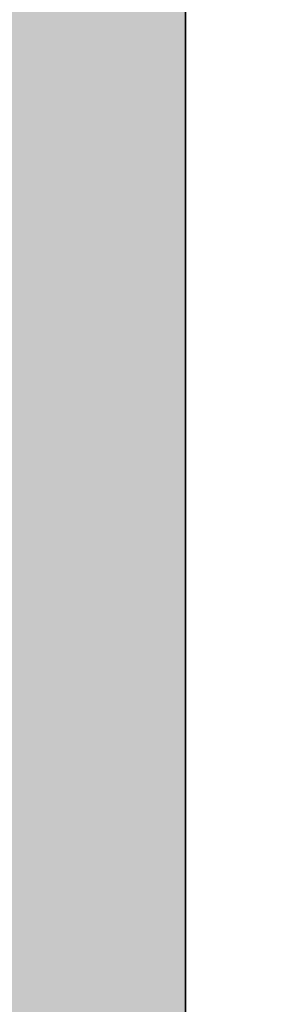
# Model space of a CAD drawing. Units: inches. Extents: x 2083 to 3317, y 1141 to 2115.
# Tile 166 of 256: x 3126.959398 to 3126.959975, y 1263.263648 to 1263.265937. Entities that reach past the tile are written whole.
import ezdxf

# ---------------------------------------------------------------- set-up
doc = ezdxf.new("R2010")
doc.units = ezdxf.units.IN
doc.layers.add('A-ANNO-DIMS', color=2, linetype='Continuous', lineweight=18)
doc.layers.add('A-WALL', color=7, linetype='Continuous', lineweight=35)
doc.layers.add('A-WALL-PATT', color=251, linetype='Continuous', lineweight=13, true_color=0x636466)
doc.styles.get("Standard").update_dxf_attribs({"font": 'arial.ttf'})
doc.dimstyles.new('ISO-25', dxfattribs={"dimtxt": 12, "dimasz": 12, "dimexe": 1.25, "dimexo": 0.625, "dimtad": 1, "dimlunit": 3, "dimtxsty": 'Standard', "dimcen": 2.5, "dimadec": 0, "dimazin": 0, "dimtfac": 1, "dimtmove": 0, "dimatfit": 3, "dimfxl": 1, "dimarcsym": 0})

# ---------------------------------------------------------------- blocks, each defined once
blk = doc.blocks.new('*D9')
at = {"layer": 'A-ANNO-DIMS', "color": 0, "lineweight": -2, "transparency": 16777216}
for p, q in [((3127.5847832, 1486.7613601), (3190.4030896, 1486.7613601)), ((3189.1530896, 1474.7613601), (3189.1530896, 1275.2613601)), ((3127.5847832, 1263.2613601), (3190.4030896, 1263.2613601))]:
    blk.add_line(p, q, dxfattribs=at)
at = {"layer": 'A-ANNO-DIMS', "color": 0, "transparency": 16777216}
for points in [[(3187.1530896, 1474.7613601), (3191.1530896, 1474.7613601), (3189.1530896, 1486.7613601)], [(3187.1530896, 1275.2613601), (3191.1530896, 1275.2613601), (3189.1530896, 1263.2613601)]]:
    blk.add_solid(points, dxfattribs=at)
at = {"layer": 'Defpoints', "color": 0, "transparency": 16777216}
for p in [(3126.9597832, 1486.7613601), (3126.9597832, 1263.2613601), (3189.1530896, 1263.2613601)]:
    blk.add_point(p, dxfattribs=at)
at = {"layer": 'A-ANNO-DIMS', "color": 0, "transparency": 16777216, "insert": (3182.4012138, 1375.0113601), "char_height": 12, "attachment_point": 5, "rotation": 90}
blk.add_mtext('18\'-7.5"', dxfattribs=at)

msp = doc.modelspace()

# ---------------------------------------------------------------- hatches: boundary and pattern name
at = {"layer": 'A-WALL-PATT'}
h = msp.add_hatch(color=256, dxfattribs=at)
h.dxf.hatch_style = 1
h.paths.add_polyline_path([(3126.9597832, 2020.7613601), (2748.9597832, 2020.7613601), (2604.9597832, 2020.7613601), (2226.9597832, 2020.7613601), (2226.9597832, 1702.7613601), (2466.9597832, 1702.7613601), (2466.9597832, 1582.7613601), (2418.9597832, 1582.7613601), (2418.9597832, 1477.7613601), (2226.9597832, 1477.7613601), (2226.9597832, 1263.2613601), (2544.9597832, 1263.2613601), (2544.9597832, 1411.7613601), (2604.9597832, 1411.7613601), (2685.9597832, 1411.7613601), (2685.9597832, 1420.7613601), (2604.9597832, 1420.7613601), (2604.9597832, 1573.7613601), (2604.9597832, 1702.7613601), (2604.9597832, 2011.7613601), (2748.9597832, 2011.7613601), (2748.9597832, 1702.7613601), (2862.9597832, 1702.7613601), (2862.9597832, 1621.7613601), (2871.9597832, 1621.7613601), (2871.9597832, 1702.7613601), (2883.9597832, 1702.7613601), (2883.9597832, 1706.9394595, -0.026459), (2883.9597832, 1711.7613601), (2757.9597832, 1711.7613601), (2757.9597832, 1807.7613601), (2787.9597832, 1807.7613601), (2787.9597832, 1812.2613601), (2757.9597832, 1812.2613601), (2757.9597832, 2011.7613601), (2877.9597832, 2011.7613601), (2877.9597832, 1812.2613601), (2847.9597832, 1812.2613601), (2847.9597832, 1807.7613601), (2889.8357425, 1807.7613601), (2889.8357425, 1812.2613601), (2882.4597832, 1812.2613601), (2882.4597832, 2011.7613601), (3117.9597832, 2011.7613601), (3117.9597832, 1812.2613601), (2937.8357425, 1812.2613601), (2937.8357425, 1807.7613601), (2995.7097832, 1807.7613601), (2995.7097832, 1796.1176655), (3000.2097832, 1796.1176655), (3000.2097832, 1807.7613601), (3117.9597832, 1807.7613601), (3117.9597832, 1711.7613601), (3000.2097832, 1711.7613601), (3000.2097832, 1760.1176655), (2998.5727047, 1760.1176655, -0.020711), (2995.7097832, 1760.1176655), (2995.7097832, 1711.7613601), (2931.9597832, 1711.7613601), (2931.9597832, 1702.7613601), (3126.9597832, 1702.7613601)])
h.paths.add_polyline_path([(2471.4597832, 2011.7613601), (2471.4597832, 1810.0113601), (2462.7169357, 1810.0113601), (2462.7169357, 1805.5113601), (2505.9597832, 1805.5113601), (2505.9597832, 1810.0113601), (2475.9597832, 1810.0113601), (2475.9597832, 2011.7613601), (2595.9597832, 2011.7613601), (2595.9597832, 1810.0113601), (2565.9597832, 1810.0113601), (2565.9597832, 1805.5113601), (2595.9597832, 1805.5113601), (2595.9597832, 1711.7613601), (2235.9597832, 1711.7613601), (2235.9597832, 1805.5113601), (2353.7097832, 1805.5113601), (2353.7097832, 1796.0541624), (2358.2097832, 1796.0541624), (2358.2097832, 1805.5113601), (2414.7169357, 1805.5113601), (2414.7169357, 1810.0113601), (2235.9597832, 1810.0113601), (2235.9597832, 2011.7613601)], flags=16)
h.paths.add_polyline_path([(2270.2047343, 1994.6100082), (2270.2047343, 1970.6100082), (2246.2047343, 1970.6100082), (2246.2047343, 1994.6100082)], flags=0)
edge = h.paths.add_edge_path(flags=0)
edge.add_ellipse((2332.027391, 1899.7981761), major_axis=(-3.0429938, 3.0429938), ratio=0.16825245, start_angle=-161.3321656, end_angle=-156.3071136, ccw=False)
edge.add_ellipse((2333.0820373, 1898.7435297), major_axis=(-1.0546463, 1.0546463), ratio=0.453532097, start_angle=-123.371019, end_angle=-94.1591066)
edge = h.paths.add_edge_path(flags=0)
edge.add_ellipse((2332.027391, 1968.8762897), major_axis=(3.0429938, 3.0429938), ratio=0.16825245, start_angle=18.6678344, end_angle=23.6928864)
edge.add_spline(control_points=[(2332.9255964, 1970.6911045), (2332.2267681, 1970.3360997), (2330.8937087, 1969.6589054), (2328.4130803, 1970.9321376), (2327.2039345, 1967.7487119), (2324.7095965, 1969.9555886), (2322.5328223, 1967.012354), (2320.0128462, 1971.2958124), (2317.6803077, 1968.1578449), (2316.0405263, 1967.1020468), (2315.4269045, 1966.8096022)], knot_values=[0, 0, 0, 0, 2.267059, 4.324559, 6.685584, 8.878641, 11.121502, 14.300359, 17.755284, 19.732645, 19.732645, 19.732645, 19.732645], degree=3, periodic=0)
edge.add_ellipse((2332.027391, 1968.8762897), major_axis=(3.0429938, 3.0429938), ratio=0.16825245, start_angle=18.6678344, end_angle=23.6928864, ccw=False)
edge.add_ellipse((2333.0820373, 1969.930936), major_axis=(1.0546463, 1.0546463), ratio=0.453532097, start_angle=56.628981, end_angle=85.8408934, ccw=False)
edge = h.paths.add_edge_path(flags=0)
edge.add_spline(control_points=[(2296.4282874, 1967.9879081), (2293.6278045, 1965.3363137), (2287.7036238, 1959.727094), (2299.7438601, 1949.9956993), (2294.5325909, 1935.6685275), (2290.5732281, 1920.6035119), (2293.3941244, 1909.9736911), (2296.1854073, 1904.9665431)], knot_values=[0.099185, 0.099185, 0.099185, 0.099185, 0.345301, 0.619822, 0.982653, 1.386093, 1.810555, 1.810555, 1.810555, 1.810555], degree=3, periodic=0)
edge.add_spline(control_points=[(2296.1854073, 1904.9665431), (2297.3835817, 1902.6193002), (2298.0009694, 1901.9493116), (2298.5529698, 1901.4681549)], knot_values=[0.006246, 0.006246, 0.006246, 0.006246, 0.055476, 0.055476, 0.055476, 0.055476], degree=3, periodic=0)
edge.add_spline(control_points=[(2298.5529698, 1901.4681549), (2297.2586121, 1900.9232238), (2295.2252939, 1900.2321257), (2293.0602287, 1900.6142053), (2292.1014227, 1900.788415), (2292.0895776, 1900.790568)], knot_values=[0.312835, 0.312835, 0.312835, 0.312835, 0.40178, 0.474987, 0.475903, 0.475903, 0.475903, 0.475903], degree=3, periodic=0)
edge.add_arc((2292.7936464, 1904.6641088), 3.9370079, 215.4208969, 259.6981795, ccw=False)
edge.add_spline(control_points=[(2289.5853139, 1902.3823039), (2289.4766524, 1902.5350874), (2289.3684805, 1902.6880353), (2289.2608648, 1902.8411699)], knot_values=[0.102872, 0.102872, 0.102872, 0.102872, 0.116896, 0.116896, 0.116896, 0.116896], degree=3, periodic=0)
edge.add_spline(control_points=[(2289.2608648, 1902.8411699), (2288.6866042, 1902.5501922), (2287.6400477, 1902.0199025), (2285.8813368, 1901.8739536), (2283.8529717, 1901.5043521), (2281.7199871, 1899.7105375), (2278.4669913, 1899.492942), (2276.1571361, 1901.8832022), (2272.2589526, 1899.8040711), (2267.7776054, 1901.8431828), (2262.2438819, 1900.1840326), (2257.414927, 1901.7820606), (2254.318374, 1900.7261196), (2253.1782849, 1900.3373431)], knot_values=[0, 0, 0, 0, 1.907977, 3.477176, 5.261074, 7.972851, 11.680248, 13.717921, 16.939592, 22.789562, 27.502503, 33.595215, 37.145618, 37.145618, 37.145618, 37.145618], degree=3, periodic=0)
edge.add_line((2253.1782849, 1900.3373431), (2250.2442397, 1902.8411699))
edge.add_line((2250.2442397, 1902.8411699), (2250.2442397, 1965.8332959))
edge.add_line((2250.2442397, 1965.8332959), (2253.1782849, 1968.3371226))
edge.add_spline(control_points=[(2253.1782849, 1968.3371226), (2254.318374, 1967.9483462), (2257.414927, 1966.8924051), (2262.2438819, 1968.4904332), (2267.7776054, 1966.8312829), (2271.5267301, 1968.5372172), (2273.8759143, 1967.8282895), (2274.2067012, 1967.7276424)], knot_values=[0, 0, 0, 0, 0.09018, 0.244935, 0.364644, 0.513233, 0.537855, 0.537855, 0.537855, 0.537855], degree=3, periodic=0)
edge.add_arc((2274.3528869, 1963.7933495), 3.9370079, 72.0511336, 92.1279492, ccw=False)
edge.add_arc((2281.2969331, 1985.2300027), 18.5962982, 252.05113361, 288.56572166)
edge.add_arc((2292.3167172, 1956.0288805), 12.6460805, 71.02678788, 113.77821843, ccw=False)
edge = h.paths.add_edge_path(flags=0)
edge.add_spline(control_points=[(2274.8994147, 1951.8561946), (2275.066156, 1951.6165924), (2275.2326866, 1951.3765878), (2275.3979871, 1951.1358545)], knot_values=[1.409916, 1.409916, 1.409916, 1.409916, 1.43159, 1.43159, 1.43159, 1.43159], degree=3, periodic=0)
edge.add_spline(control_points=[(2275.3979871, 1951.1358545), (2275.7921055, 1950.5618854), (2276.1792311, 1949.9837745), (2276.5455462, 1949.3971029)], knot_values=[1.358238, 1.358238, 1.358238, 1.358238, 1.409916, 1.409916, 1.409916, 1.409916], degree=3, periodic=0)
edge.add_line((2276.5455462, 1949.3971029), (2277.437289, 1947.8621847))
edge.add_spline(control_points=[(2277.437289, 1947.8621847), (2276.3038341, 1945.6731147), (2274.6396979, 1942.4268817), (2274.631615, 1938.0938998), (2272.7991237, 1930.8515498), (2274.3564261, 1943.8970461), (2275.9476814, 1947.9233558), (2276.5455462, 1949.3971029)], knot_values=[0.005632, 0.005632, 0.005632, 0.005632, 0.186014, 0.266002, 0.357087, 0.59639, 0.739732, 0.739732, 0.739732, 0.739732], degree=3, periodic=0)
edge.add_spline(control_points=[(2276.5455462, 1949.3971029), (2276.1792311, 1949.9837745), (2275.7921055, 1950.5618854), (2275.3979871, 1951.1358545)], knot_values=[1.358238, 1.358238, 1.358238, 1.358238, 1.409916, 1.409916, 1.409916, 1.409916], degree=3, periodic=0)
edge.add_spline(control_points=[(2275.3979871, 1951.1358545), (2274.9425002, 1950.0804523), (2274.2077604, 1948.0252718), (2273.9346018, 1944.8514774), (2272.4685341, 1937.6274891), (2273.4662155, 1945.6964663), (2274.7006154, 1951.0594725), (2274.8994147, 1951.8561946)], knot_values=[0.104364, 0.104364, 0.104364, 0.104364, 0.189636, 0.269624, 0.36071, 0.600013, 0.644622, 0.644622, 0.644622, 0.644622], degree=3, periodic=0)
h.paths.add_polyline_path([(2269.1675139, 1963.1275729, -0.357527), (2268.170633, 1960.9763695, -0.092561), (2268.170633, 1939.4363249, -0.357527), (2269.1675139, 1937.2851215, -0.357527), (2267.0163105, 1938.2820024, -0.164785), (2254.6855813, 1938.2820024, -0.357527), (2252.5343779, 1937.2851215, -0.357527), (2253.5312587, 1939.4363249, -0.092561), (2253.5312587, 1960.9763695, -0.357527), (2252.5343779, 1963.1275729, -0.357527), (2254.6855813, 1962.130692, -0.164785), (2267.0163105, 1962.130692, -0.357527)], flags=0)
h.paths.add_polyline_path([(2248.8740679, 1967.8017998), (2248.8740679, 1957.0277095), (2249.4577833, 1957.0277095), (2249.4577833, 1911.6467562), (2248.8740679, 1911.6467562), (2248.8740679, 1900.8726659), (2246.5118632, 1900.8726659, 0.197327), (2244.1496584, 1902.4568734), (2244.1496584, 1966.2175923, 0.197327), (2246.5118632, 1967.8017998)], flags=0)
h.paths.add_polyline_path([(2269.1675139, 1931.3893442, -0.357527), (2268.170633, 1929.2381408, -0.092561), (2268.170633, 1907.6980962, -0.357527), (2269.1675139, 1905.5468928, -0.357527), (2267.0163105, 1906.5437737, -0.164785), (2254.6855813, 1906.5437737, -0.357527), (2252.5343779, 1905.5468928, -0.357527), (2253.5312587, 1907.6980962, -0.092561), (2253.5312587, 1929.2381408, -0.357527), (2252.5343779, 1931.3893442, -0.357527), (2254.6855813, 1930.3924634, -0.164785), (2267.0163105, 1930.3924634, -0.357527)], flags=0)
edge = h.paths.add_edge_path(flags=0)
edge.add_spline(control_points=[(2276.1968578, 1906.7237016), (2276.1681442, 1909.0289278), (2276.1140492, 1913.371852), (2270.5984171, 1924.9249783), (2273.9051746, 1919.0127787), (2275.9217115, 1916.2620626), (2275.4745699, 1912.4021495), (2277.2578735, 1910.3806206), (2276.6960436, 1908.2250358), (2276.6462176, 1906.8130226), (2276.6178249, 1906.0084068)], knot_values=[0, 0, 0, 0, 8.61026, 16.221274, 18.843057, 23.804898, 27.440828, 29.356102, 31.203478, 33.650687, 33.650687, 33.650687, 33.650687], degree=3, periodic=0)
edge.add_spline(control_points=[(2276.6178249, 1906.0084068), (2276.6233131, 1905.6241436), (2276.4977381, 1904.6286608), (2275.4417789, 1903.8547251), (2274.9373144, 1903.0804497), (2274.8590804, 1902.8411699)], knot_values=[0.156488, 0.156488, 0.156488, 0.156488, 0.184398, 0.231376, 0.250598, 0.250598, 0.250598, 0.250598], degree=3, periodic=0)
edge.add_line((2274.8590804, 1902.8411699), (2276.50598, 1902.8411699))
edge.add_spline(control_points=[(2276.50598, 1902.8411699), (2276.7883084, 1903.0849395), (2277.6650711, 1904.1251958), (2278.2495378, 1904.340738), (2277.6538719, 1908.5273866), (2278.15567, 1906.2278078), (2278.100464, 1905.2859484), (2278.8466748, 1904.0690054), (2277.8567853, 1903.4149482), (2277.8741909, 1902.9910497), (2277.9035616, 1902.8411699)], knot_values=[0.059574, 0.059574, 0.059574, 0.059574, 0.080753, 0.103741, 0.16972, 0.176036, 0.207137, 0.240474, 0.262341, 0.27366, 0.27366, 0.27366, 0.27366], degree=3, periodic=0)
edge.add_line((2277.9035616, 1902.8411699), (2280.0298255, 1902.8411699))
edge.add_spline(control_points=[(2280.0298255, 1902.8411699), (2279.8882214, 1903.088398), (2279.4992571, 1903.9815512), (2280.1522839, 1905.9393491), (2278.103615, 1909.6577572), (2279.7623946, 1907.185285), (2280.3279002, 1904.8748608), (2280.4851086, 1903.4895904), (2281.4632687, 1903.2494323), (2281.7583431, 1902.9364967), (2281.8340361, 1902.8411699)], knot_values=[0.013856, 0.013856, 0.013856, 0.013856, 0.034874, 0.088867, 0.107879, 0.126738, 0.158714, 0.193757, 0.217487, 0.226722, 0.226722, 0.226722, 0.226722], degree=3, periodic=0)
edge.add_spline(control_points=[(2281.8340361, 1902.8411699), (2281.7875348, 1902.8267029), (2281.6470224, 1902.7829881), (2281.3955272, 1902.85949), (2281.088077, 1902.9852418), (2280.7206826, 1903.060902), (2280.3334513, 1903.0257257), (2280.1247668, 1902.898879), (2280.0298255, 1902.8411699)], knot_values=[0, 0, 0, 0, 0.14413, 0.435517, 0.749276, 1.153046, 1.548371, 1.878348, 1.878348, 1.878348, 1.878348], degree=3, periodic=0)
edge.add_line((2280.0298255, 1902.8411699), (2277.9035616, 1902.8411699))
edge.add_spline(control_points=[(2277.9035616, 1902.8411699), (2277.892855, 1902.7958553), (2277.865396, 1902.6796374), (2277.6074793, 1902.6874828), (2277.2740503, 1902.8006999), (2276.8379209, 1902.6197745), (2276.5838074, 1902.7892611), (2276.50598, 1902.8411699)], knot_values=[0, 0, 0, 0, 0.127189, 0.326199, 0.628009, 1.24357, 1.515331, 1.515331, 1.515331, 1.515331], degree=3, periodic=0)
edge.add_line((2276.50598, 1902.8411699), (2274.8590804, 1902.8411699))
edge.add_spline(control_points=[(2274.8590804, 1902.8411699), (2274.8144367, 1902.8985868), (2274.7251297, 1903.013446), (2274.4934765, 1903.1189684), (2274.2442854, 1902.9605386), (2273.9371207, 1903.1849416), (2273.6140395, 1902.9831428), (2273.4083164, 1902.8830449), (2273.322254, 1902.8411699)], knot_values=[0, 0, 0, 0, 0.21843, 0.436957, 0.687977, 0.990379, 1.398396, 1.69185, 1.69185, 1.69185, 1.69185], degree=3, periodic=0)
edge.add_spline(control_points=[(2273.322254, 1902.8411699), (2273.6167403, 1903.445692), (2274.2739977, 1904.5382529), (2276.0272387, 1904.5737017), (2276.2069634, 1906.5836372), (2276.1968578, 1906.7237016)], knot_values=[0.012227, 0.012227, 0.012227, 0.012227, 0.059472, 0.106218, 0.134458, 0.134458, 0.134458, 0.134458], degree=3, periodic=0)
h.paths.add_polyline_path([(2270.7760538, 1897.7898284), (2270.7760538, 1873.7898284), (2246.7760538, 1873.7898284), (2246.7760538, 1897.7898284)], flags=0)
h.paths.add_polyline_path([(2353.7097832, 1760.0050593), (2353.7097832, 1760.0541624), (2358.2097832, 1760.0541624, -0.033729)], flags=0)
h.paths.add_polyline_path([(2321.8191188, 1737.5291862), (2341.9953271, 1737.5291862, -0.414214), (2343.2032727, 1736.3212406), (2343.2032727, 1721.0205964, -0.414214), (2341.9953271, 1719.8126508), (2321.8191188, 1719.8126508, -0.414214), (2320.6111732, 1721.0205964), (2320.6111732, 1736.3212406, -0.414214)], flags=0)
h.paths.add_polyline_path([(2324.2350099, 1736.3212406), (2339.5794359, 1736.3212406, -0.414214), (2341.9953271, 1733.9053494), (2341.9953271, 1725.4497302, -0.414214), (2339.5794359, 1723.033839), (2333.6805885, 1723.033839), (2333.8453172, 1722.0454666, -0.870646), (2335.4253988, 1721.8258934, -0.767327), (2333.922694, 1721.4232449), (2331.2910241, 1721.4232449, -0.767327), (2329.7883193, 1721.8258934, -0.870646), (2331.3684009, 1722.0454666), (2331.5331296, 1723.033839), (2324.2350099, 1723.033839, -0.414214), (2321.8191188, 1725.4497302), (2321.8191188, 1733.9053494, -0.414214)], flags=0)
h.paths.add_polyline_path([(2570.4837892, 1928.6154443), (2589.6837892, 1928.6154443), (2590.1688286, 1928.6154443), (2590.1688286, 1904.9933971), (2570.4837892, 1904.9933971)], flags=0)
h.paths.add_polyline_path([(2574.4473242, 1927.2638215, -1), (2572.8288357, 1927.2638215, -1)], flags=0)
h.paths.add_polyline_path([(2573.0898665, 1926.9408768), (2573.925032, 1927.7760423), (2574.1477428, 1927.5533315), (2573.3125773, 1926.718166)], flags=0)
h.paths.add_polyline_path([(2578.7790648, 1919.7296175, -1), (2571.5916632, 1919.7296175, -1)], flags=0)
h.paths.add_polyline_path([(2578.385364, 1919.7296175, -1), (2571.985364, 1919.7296175, -1)], flags=0)
h.paths.add_polyline_path([(2331.5957638, 1729.4762156, -1), (2333.6179542, 1729.4762156, -1)], flags=0)
h.paths.add_polyline_path([(2578.0342282, 1927.2638215, -1), (2576.4157396, 1927.2638215, -1)], flags=0)
h.paths.add_polyline_path([(2576.6888513, 1927.5310886), (2576.9115621, 1927.7537993), (2577.7467276, 1926.9186339), (2577.5240168, 1926.6959231)], flags=0)
h.paths.add_polyline_path([(2578.1390648, 1909.8595388, -1), (2572.2316632, 1909.8595388, -1)], flags=0)
h.paths.add_polyline_path([(2577.745364, 1909.8595388, -1), (2572.625364, 1909.8595388, -1)], flags=0)
h.paths.add_polyline_path([(2583.7977179, 1927.2638215, -1), (2582.1792294, 1927.2638215, -1)], flags=0)
h.paths.add_polyline_path([(2582.7186487, 1927.7537993), (2583.5538142, 1926.9186339), (2583.3311034, 1926.6959231), (2582.4959379, 1927.5310886)], flags=0)
h.paths.add_polyline_path([(2582.4959379, 1927.5310886), (2582.7186487, 1927.7537993), (2583.5538142, 1926.9186339), (2583.3311034, 1926.6959231)], flags=0)
h.paths.add_polyline_path([(2587.7390648, 1920.5296175, -1), (2581.8316632, 1920.5296175, -1)], flags=0)
h.paths.add_polyline_path([(2587.345364, 1920.5296175, -1), (2582.225364, 1920.5296175, -1)], flags=0)
h.paths.add_polyline_path([(2587.3846219, 1927.2638215, -1), (2585.7661333, 1927.2638215, -1)], flags=0)
h.paths.add_polyline_path([(2586.0819925, 1926.9802469), (2586.917158, 1927.8154124), (2587.1398688, 1927.5927016), (2586.3047033, 1926.7575361)], flags=0)
h.paths.add_polyline_path([(2588.3790648, 1910.6595388, -1), (2581.1916632, 1910.6595388, -1)], flags=0)
h.paths.add_polyline_path([(2587.985364, 1910.6595388, -1), (2581.585364, 1910.6595388, -1)], flags=0)
h.paths.add_polyline_path([(2417.1677288, 1729.4778955), (2437.3439372, 1729.4778955, -0.414214), (2438.5518828, 1728.2699499), (2438.5518828, 1712.9693057, -0.414214), (2437.3439372, 1711.7613601), (2417.1677288, 1711.7613601, -0.414214), (2415.9597832, 1712.9693057), (2415.9597832, 1728.2699499, -0.414214)], flags=0)
h.paths.add_polyline_path([(2419.58362, 1728.2699499), (2434.928046, 1728.2699499, -0.414214), (2437.3439372, 1725.8540587), (2437.3439372, 1717.3984395, -0.414214), (2434.928046, 1714.9825483), (2429.0291985, 1714.9825483), (2429.1939273, 1713.9941758, -0.870646), (2430.7740089, 1713.7746027, -0.767327), (2429.2713041, 1713.3719542), (2426.6396342, 1713.3719542, -0.767327), (2425.1369294, 1713.7746027, -0.870646), (2426.717011, 1713.9941758), (2426.8817397, 1714.9825483), (2419.58362, 1714.9825483, -0.414214), (2417.1677288, 1717.3984395), (2417.1677288, 1725.8540587, -0.414214)], flags=0)
h.paths.add_polyline_path([(2419.58362, 1728.2699499), (2434.928046, 1728.2699499, -0.414214), (2437.3439372, 1725.8540587), (2437.3439372, 1717.3984395, -0.414214), (2434.928046, 1714.9825483), (2429.0291985, 1714.9825483), (2428.3581177, 1719.0090337), (2427.5528206, 1719.0090337), (2426.8817397, 1714.9825483), (2419.58362, 1714.9825483, -0.414214), (2417.1677288, 1717.3984395), (2417.1677288, 1725.8540587, -0.414214)], flags=0)
h.paths.add_polyline_path([(2426.9443739, 1721.4249248, -1), (2428.9665643, 1721.4249248, -1)], flags=0)
h.paths.add_polyline_path([(2475.9597832, 1702.7613601), (2595.9597832, 1702.7613601), (2595.9597832, 1582.7613601), (2475.9597832, 1582.7613601)], flags=16)
h.paths.add_polyline_path([(2427.9597832, 1573.7613601), (2595.9597832, 1573.7613601), (2595.9597832, 1468.7613601), (2595.9597832, 1420.7613601), (2384.4597832, 1420.7613601), (2384.4597832, 1468.7613601), (2427.9597832, 1468.7613601)], flags=16)
h.paths.add_polyline_path([(2379.9597832, 1468.7613601), (2379.9597832, 1420.7613601), (2235.9597832, 1420.7613601), (2235.9597832, 1468.7613601)], flags=16)
h.paths.add_polyline_path([(2317.8159962, 1466.695767), (2337.9922045, 1466.695767, -0.414214), (2339.2001501, 1465.4878214), (2339.2001501, 1450.1871771, -0.414214), (2337.9922045, 1448.9792315), (2317.8159962, 1448.9792315, -0.414214), (2316.6080506, 1450.1871771), (2316.6080506, 1465.4878214, -0.414214)], flags=0)
h.paths.add_polyline_path([(2320.2318874, 1465.4878214), (2335.5763133, 1465.4878214, -0.414214), (2337.9922045, 1463.0719302), (2337.9922045, 1454.616311, -0.414214), (2335.5763133, 1452.2004198), (2329.6774659, 1452.2004198), (2329.8421946, 1451.2120473, -0.870646), (2331.4222762, 1450.9924742, -0.767327), (2329.9195714, 1450.5898257), (2327.2879015, 1450.5898257, -0.767327), (2325.7851967, 1450.9924742, -0.870646), (2327.3652783, 1451.2120473), (2327.530007, 1452.2004198), (2320.2318874, 1452.2004198, -0.414214), (2317.8159962, 1454.616311), (2317.8159962, 1463.0719302, -0.414214)], flags=0)
h.paths.add_polyline_path([(2320.2318874, 1465.4878214), (2335.5763133, 1465.4878214, -0.414214), (2337.9922045, 1463.0719302), (2337.9922045, 1454.616311, -0.414214), (2335.5763133, 1452.2004198), (2329.6774659, 1452.2004198), (2329.006385, 1456.2269051), (2328.2010879, 1456.2269051), (2327.530007, 1452.2004198), (2320.2318874, 1452.2004198, -0.414214), (2317.8159962, 1454.616311), (2317.8159962, 1463.0719302, -0.414214)], flags=0)
h.paths.add_polyline_path([(2327.5926413, 1458.6427963, -1), (2329.6148317, 1458.6427963, -1)], flags=0)
h.paths.add_polyline_path([(2244.4117436, 1433.3404531), (2241.9209449, 1433.3404531, -0.414214), (2240.0178562, 1435.2435418), (2240.0178562, 1440.9528078, -0.414211), (2241.920925, 1442.8558965), (2244.4117436, 1442.8558965, -1.976472)], flags=0)
h.paths.add_polyline_path([(2245.3568884, 1434.3975358, -0.414214), (2245.3568884, 1441.7988138, -2.144098)], flags=0)
h.paths.add_polyline_path([(2535.9597832, 1416.2613601), (2535.9597832, 1272.2613601), (2235.9597832, 1272.2613601), (2235.9597832, 1416.2613601)], flags=16)
h.paths.add_polyline_path([(2260.1195614, 1384.2928413), (2260.1195614, 1362.0386487), (2237.8653688, 1362.0386487), (2237.8653688, 1384.2928413)], flags=0)
edge = h.paths.add_edge_path(flags=0)
edge.add_line((2318.2518466, 1362.0932983), (2318.1457968, 1362.0009726))
edge.add_ellipse((2317.4451158, 1360.4310442), major_axis=(2.8216404, 2.8216404), ratio=0.16825245, start_angle=18.6678344, end_angle=20.9481273, ccw=False)
edge.add_ellipse((2318.4230451, 1361.4089735), major_axis=(0.9779293, 0.9779293), ratio=0.453532097, start_angle=56.628981, end_angle=70.2262012, ccw=False)
edge = h.paths.add_edge_path(flags=0)
edge.add_line((2319.1073699, 1295.5710784), (2319.0150442, 1295.6771282))
edge.add_ellipse((2317.4451158, 1296.3778091), major_axis=(-2.8216404, 2.8216404), ratio=0.16825245, start_angle=-161.3321656, end_angle=-159.0518727, ccw=False)
edge.add_ellipse((2318.4230451, 1295.3998798), major_axis=(-0.9779293, 0.9779293), ratio=0.453532097, start_angle=-123.371019, end_angle=-109.7737988)
edge = h.paths.add_edge_path(flags=0)
edge.add_spline(control_points=[(2284.2103489, 1301.1702189), (2284.5806878, 1300.444719), (2284.8911891, 1299.8920243), (2285.159553, 1299.4610182)], knot_values=[0.039066, 0.039066, 0.039066, 0.039066, 0.055476, 0.055476, 0.055476, 0.055476], degree=3, periodic=0)
edge.add_line((2285.159553, 1299.4610182), (2284.2103489, 1301.1702189))
edge = h.paths.add_edge_path(flags=0)
edge.add_line((2280.4124579, 1297.2980125), (2283.3699905, 1297.0361216))
edge.add_line((2283.3699905, 1297.0361216), (2286.4056902, 1297.9263104))
edge.add_spline(control_points=[(2286.4056902, 1297.9263104), (2285.305487, 1297.4631193), (2284.3447774, 1297.1291508), (2283.3699905, 1297.0361216)], knot_values=[0.394369, 0.394369, 0.394369, 0.394369, 0.475903, 0.475903, 0.475903, 0.475903], degree=3, periodic=0)
edge.add_spline(control_points=[(2283.3699905, 1297.0361216), (2283.2813895, 1297.027666), (2282.316289, 1296.9573356), (2281.3125019, 1297.1344787), (2280.4234414, 1297.2960161), (2280.4124579, 1297.2980125)], knot_values=[0.312835, 0.312835, 0.312835, 0.312835, 0.320246, 0.393453, 0.394369, 0.394369, 0.394369, 0.394369], degree=3, periodic=0)
edge = h.paths.add_edge_path(flags=0)
edge.add_line((2284.4355615, 1359.6072854), (2280.4462909, 1355.328047))
edge.add_line((2280.4462909, 1355.328047), (2279.5799868, 1351.0177544))
edge.add_line((2279.5799868, 1351.0177544), (2282.4129737, 1346.5804327))
edge.add_spline(control_points=[(2282.4129737, 1346.5804327), (2283.1533308, 1345.5892358), (2284.2528957, 1344.0288973), (2284.801037, 1342.3871671), (2284.9351625, 1341.8055443)], knot_values=[1.240098, 1.240098, 1.240098, 1.240098, 1.332892, 1.382712, 1.382712, 1.382712, 1.382712], degree=3, periodic=0)
edge.add_spline(control_points=[(2284.9351625, 1341.8055443), (2285.3191079, 1340.1406002), (2285.2330291, 1338.4092041), (2284.9099384, 1336.6541222)], knot_values=[1.097484, 1.097484, 1.097484, 1.097484, 1.240098, 1.240098, 1.240098, 1.240098], degree=3, periodic=0)
edge.add_spline(control_points=[(2284.9099384, 1336.6541222), (2284.5868478, 1334.8990403), (2284.0267453, 1333.1202725), (2283.4626437, 1331.3605849)], knot_values=[0.95487, 0.95487, 0.95487, 0.95487, 1.097484, 1.097484, 1.097484, 1.097484], degree=3, periodic=0)
edge.add_line((2283.4626437, 1331.3605849), (2281.8903759, 1326.153357))
edge.add_line((2281.8903759, 1326.153357), (2280.7562592, 1321.0560888))
edge.add_line((2280.7562592, 1321.0560888), (2280.2992048, 1316.0019772))
edge.add_line((2280.2992048, 1316.0019772), (2280.7159327, 1310.9500678))
edge.add_line((2280.7159327, 1310.9500678), (2282.0280939, 1305.9721367))
edge.add_line((2282.0280939, 1305.9721367), (2284.2103489, 1301.1702189))
edge.add_spline(control_points=[(2284.2103489, 1301.1702189), (2283.3407305, 1302.7301854), (2282.6119044, 1304.3364933), (2282.0280939, 1305.9721367)], knot_values=[0.099185, 0.099185, 0.099185, 0.099185, 0.241799, 0.241799, 0.241799, 0.241799], degree=3, periodic=0)
edge.add_spline(control_points=[(2282.0280939, 1305.9721367), (2281.4442835, 1307.6077801), (2281.0054886, 1309.2727591), (2280.7159327, 1310.9500678)], knot_values=[0.241799, 0.241799, 0.241799, 0.241799, 0.384413, 0.384413, 0.384413, 0.384413], degree=3, periodic=0)
edge.add_spline(control_points=[(2280.7159327, 1310.9500678), (2280.4332411, 1312.5876134), (2280.2893863, 1314.2769594), (2280.2988938, 1315.9620324), (2280.2992048, 1316.0019772)], knot_values=[0.384413, 0.384413, 0.384413, 0.384413, 0.523647, 0.527028, 0.527028, 0.527028, 0.527028], degree=3, periodic=0)
edge.add_spline(control_points=[(2280.2992048, 1316.0019772), (2280.3123257, 1317.6869552), (2280.4778706, 1319.3679256), (2280.7562592, 1321.0560888)], knot_values=[0.527028, 0.527028, 0.527028, 0.527028, 0.669642, 0.669642, 0.669642, 0.669642], degree=3, periodic=0)
edge.add_spline(control_points=[(2280.7562592, 1321.0560888), (2281.0346478, 1322.7442519), (2281.4258801, 1324.4396079), (2281.8903759, 1326.153357)], knot_values=[0.669642, 0.669642, 0.669642, 0.669642, 0.812256, 0.812256, 0.812256, 0.812256], degree=3, periodic=0)
edge.add_spline(control_points=[(2281.8903759, 1326.153357), (2282.2643834, 1327.5332507), (2282.7878702, 1329.2618097), (2283.352751, 1331.0177803), (2283.4626437, 1331.3605849)], knot_values=[0.812256, 0.812256, 0.812256, 0.812256, 0.927087, 0.95487, 0.95487, 0.95487, 0.95487], degree=3, periodic=0)
edge.add_line((2283.4626437, 1331.3605849), (2284.9099384, 1336.6541222))
edge.add_line((2284.9099384, 1336.6541222), (2284.9351625, 1341.8055443))
edge.add_line((2284.9351625, 1341.8055443), (2282.4129737, 1346.5804327))
edge.add_spline(control_points=[(2282.4129737, 1346.5804327), (2281.2751273, 1348.1037918), (2280.0784467, 1349.5703178), (2279.5799868, 1351.0177544)], knot_values=[1.382712, 1.382712, 1.382712, 1.382712, 1.525326, 1.525326, 1.525326, 1.525326], degree=3, periodic=0)
edge.add_spline(control_points=[(2279.5799868, 1351.0177544), (2279.4432818, 1351.4147209), (2279.1363124, 1352.856922), (2279.7351897, 1354.2903851), (2280.4462909, 1355.328047)], knot_values=[1.525326, 1.525326, 1.525326, 1.525326, 1.564439, 1.667941, 1.667941, 1.667941, 1.667941], degree=3, periodic=0)
edge.add_spline(control_points=[(2280.4462909, 1355.328047), (2281.4261132, 1356.7578354), (2282.9308373, 1358.1825604), (2284.4355615, 1359.6072854)], knot_values=[1.667941, 1.667941, 1.667941, 1.667941, 1.810555, 1.810555, 1.810555, 1.810555], degree=3, periodic=0)
edge.add_arc((2280.6230749, 1348.518181), 11.7261796, 71.02678788, 113.77821843)
edge.add_arc((2270.4048917, 1375.5951559), 17.2435667, 252.05113361, 288.56572166, ccw=False)
edge.add_arc((2263.9659692, 1355.7178471), 3.6506221, 72.0511336, 92.1279492)
edge.add_arc((2263.9659692, 1355.7178471), 3.6506221, 92.1279492, 177.98513)
edge.add_spline(control_points=[(2260.3176041, 1355.8461989), (2260.2604169, 1354.2206683), (2260.551278, 1350.1865469), (2262.9993445, 1346.7662507), (2264.4727415, 1344.6490245)], knot_values=[1.43159, 1.43159, 1.43159, 1.43159, 1.564144, 1.770695, 1.770695, 1.770695, 1.770695], degree=3, periodic=0)
edge.add_line((2264.4727415, 1344.6490245), (2264.9355904, 1343.9825301))
edge.add_spline(control_points=[(2263.8010444, 1340.2481052), (2263.8432379, 1340.5140884), (2264.0672444, 1341.7564652), (2264.5126928, 1343.0024532), (2264.9350468, 1343.9810834)], knot_values=[0.53657, 0.53657, 0.53657, 0.53657, 0.559349, 0.644622, 0.644622, 0.644622, 0.644622], degree=3, periodic=0)
edge.add_spline(control_points=[(2264.9350468, 1343.9810834), (2265.1177715, 1343.7149747), (2265.2988751, 1343.4479058), (2265.4767562, 1343.1793646)], knot_values=[1.384077, 1.384077, 1.384077, 1.384077, 1.409916, 1.409916, 1.409916, 1.409916], degree=3, periodic=0)
edge.add_spline(control_points=[(2265.4767562, 1343.1793646), (2265.6546373, 1342.9108234), (2265.8292958, 1342.64081), (2265.9991301, 1342.368812)], knot_values=[1.358238, 1.358238, 1.358238, 1.358238, 1.384077, 1.384077, 1.384077, 1.384077], degree=3, periodic=0)
edge.add_line((2265.9991301, 1342.368812), (2266.8260057, 1340.9455468))
edge.add_spline(control_points=[(2266.8260057, 1340.9455468), (2268.894401, 1337.0896912), (2271.3981727, 1325.8430009), (2270.5161644, 1310.5685568), (2275.9193759, 1301.860609), (2277.7895113, 1299.1994495)], knot_values=[0.116896, 0.116896, 0.116896, 0.116896, 0.472987, 1.050969, 1.313793, 1.313793, 1.313793, 1.313793], degree=3, periodic=0)
edge.add_spline(control_points=[(2277.7895113, 1299.1994495), (2277.8394051, 1299.1284519), (2277.8894277, 1299.0574975), (2277.9395717, 1298.9865839)], knot_values=[0.109884, 0.109884, 0.109884, 0.109884, 0.116896, 0.116896, 0.116896, 0.116896], degree=3, periodic=0)
edge.add_line((2277.9395717, 1298.9865839), (2277.7888489, 1299.1991139))
edge.add_spline(control_points=[(2277.7888489, 1299.1991139), (2277.2565819, 1298.9294144), (2276.2863504, 1298.4379024), (2275.0393517, 1298.3344186), (2274.3833299, 1298.2388951), (2274.2152543, 1298.209338)], knot_values=[33.12187, 33.12187, 33.12187, 33.12187, 35.029056, 36.598255, 37.144827, 37.144827, 37.144827, 37.144827], degree=3, periodic=0)
edge.add_line((2274.2152543, 1298.209338), (2273.073147, 1297.8929607))
edge.add_spline(control_points=[(2273.073147, 1297.8929607), (2272.3229363, 1297.579784), (2271.0391507, 1296.5105078), (2269.2483948, 1296.2260622), (2268.4231004, 1296.3746543)], knot_values=[26.532584, 26.532584, 26.532584, 26.532584, 29.198919, 31.839101, 31.839101, 31.839101, 31.839101], degree=3, periodic=0)
edge.add_line((2268.4231004, 1296.3746543), (2263.8785014, 1297.4575338))
edge.add_spline(control_points=[(2263.8785014, 1297.4575338), (2263.5560769, 1297.3594345), (2261.8603064, 1296.8386943), (2260.2387805, 1297.2824073), (2258.9334543, 1297.5164611)], knot_values=[15.919551, 15.919551, 15.919551, 15.919551, 16.939592, 21.226067, 21.226067, 21.226067, 21.226067], degree=3, periodic=0)
edge.add_line((2258.9334543, 1297.5164611), (2254.0552332, 1297.3290098))
edge.add_spline(control_points=[(2254.0552332, 1297.3290098), (2253.7555255, 1297.295815), (2252.1136834, 1297.1651738), (2250.4618687, 1297.5442209), (2249.1296862, 1297.6678818)], knot_values=[5.306517, 5.306517, 5.306517, 5.306517, 6.276435, 10.613034, 10.613034, 10.613034, 10.613034], degree=3, periodic=0)
edge.add_line((2249.1296862, 1297.6678818), (2244.3316495, 1296.8777561))
edge.add_line((2244.3316495, 1296.8777561), (2241.6110326, 1299.1994495))
edge.add_line((2241.6110326, 1299.1994495), (2241.6110326, 1357.6094038))
edge.add_line((2241.6110326, 1357.6094038), (2244.3316495, 1359.9310973))
edge.add_line((2244.3316495, 1359.9310973), (2252.7288228, 1359.5426917))
edge.add_spline(control_points=[(2252.7288228, 1359.5426917), (2252.8709387, 1359.5464396), (2253.3057402, 1359.5481716), (2253.7398447, 1359.5142744), (2254.0317419, 1359.4824261)], knot_values=[0.233291, 0.233291, 0.233291, 0.233291, 0.244935, 0.268927, 0.268927, 0.268927, 0.268927], degree=3, periodic=0)
edge.add_line((2254.0317419, 1359.4824261), (2259.5871899, 1359.4163899))
edge.add_spline(control_points=[(2259.5871899, 1359.4163899), (2260.6770676, 1359.6285026), (2262.0731971, 1359.8970025), (2263.5236925, 1359.4592776), (2263.8304173, 1359.3659518)], knot_values=[0.422516, 0.422516, 0.422516, 0.422516, 0.513233, 0.537855, 0.537855, 0.537855, 0.537855], degree=3, periodic=0)
edge.add_arc((2263.9659692, 1355.7178471), 3.6506221, 72.0511336, 92.1279492, ccw=False)
edge.add_arc((2270.4048917, 1375.5951559), 17.2435667, 252.05113361, 288.56572166)
edge.add_arc((2280.6230749, 1348.518181), 11.7261796, 71.02678788, 113.77821843, ccw=False)
h.paths.add_polyline_path([(2240.3405298, 1359.4347149), (2240.3405298, 1349.4443532), (2240.8817846, 1349.4443532), (2240.8817846, 1307.3645001), (2240.3405298, 1307.3645001), (2240.3405298, 1297.3741385), (2238.1501565, 1297.3741385, 0.197327), (2235.9597832, 1298.8431076), (2235.9597832, 1357.9657458, 0.197327), (2238.1501565, 1359.4347149)], flags=0)
h.paths.add_polyline_path([(2259.1577904, 1355.1005005, -0.357527), (2258.2334246, 1353.1057799, -0.092561), (2258.2334246, 1333.1326007, -0.357527), (2259.1577904, 1331.1378801, -0.357527), (2257.1630698, 1332.0622458, -0.164785), (2245.7293022, 1332.0622458, -0.357527), (2243.7345816, 1331.1378801, -0.357527), (2244.6589474, 1333.1326007, -0.092561), (2244.6589474, 1353.1057799, -0.357527), (2243.7345816, 1355.1005005, -0.357527), (2245.7293022, 1354.1761347, -0.164785), (2257.1630698, 1354.1761347, -0.357527)], flags=0)
edge = h.paths.add_edge_path(flags=0)
edge.add_line((2265.9991301, 1342.368812), (2266.8260057, 1340.9455468))
edge.add_line((2266.8260057, 1340.9455468), (2265.3075567, 1337.8140664))
edge.add_line((2265.3075567, 1337.8140664), (2264.358232, 1334.6529388))
edge.add_line((2264.358232, 1334.6529388), (2264.2620123, 1333.7997046))
edge.add_spline(control_points=[(2264.2620123, 1333.7997046), (2264.2083565, 1333.187055), (2264.1620602, 1332.3655252), (2264.0071444, 1331.4139326), (2263.9690487, 1331.2018338)], knot_values=[0.464444, 0.464444, 0.464444, 0.464444, 0.516691, 0.531608, 0.531608, 0.531608, 0.531608], degree=3, periodic=0)
edge.add_spline(control_points=[(2263.9690487, 1331.2018338), (2263.7745349, 1330.1188727), (2263.4243703, 1328.7908386), (2263.2574202, 1328.5306516), (2263.2340282, 1328.5146115)], knot_values=[0.372682, 0.372682, 0.372682, 0.372682, 0.44885, 0.464444, 0.464444, 0.464444, 0.464444], degree=3, periodic=0)
edge.add_spline(control_points=[(2263.2340282, 1328.5146115), (2263.096382, 1328.4202271), (2263.1311696, 1329.3014765), (2263.2749528, 1330.6157493)], knot_values=[0.280919, 0.280919, 0.280919, 0.280919, 0.372682, 0.372682, 0.372682, 0.372682], degree=3, periodic=0)
edge.add_spline(control_points=[(2263.2749528, 1330.6157493), (2263.4187361, 1331.930022), (2263.6715151, 1333.677318), (2263.9698519, 1335.3150268)], knot_values=[0.189157, 0.189157, 0.189157, 0.189157, 0.280919, 0.280919, 0.280919, 0.280919], degree=3, periodic=0)
edge.add_spline(control_points=[(2263.9698519, 1335.3150268), (2264.1004958, 1336.0321917), (2264.4187827, 1337.6219113), (2264.7548476, 1338.8644304), (2264.9474193, 1339.4911244)], knot_values=[0.097394, 0.097394, 0.097394, 0.097394, 0.137578, 0.189157, 0.189157, 0.189157, 0.189157], degree=3, periodic=0)
edge.add_spline(control_points=[(2264.9474193, 1339.4911244), (2265.2900171, 1340.6060546), (2265.6442376, 1341.4939958), (2265.9991301, 1342.368812)], knot_values=[0.005632, 0.005632, 0.005632, 0.005632, 0.097394, 0.097394, 0.097394, 0.097394], degree=3, periodic=0)
h.paths.add_polyline_path([(2259.1577904, 1325.6709733, -0.357527), (2258.2334246, 1323.6762527, -0.092561), (2258.2334246, 1303.7030735, -0.357527), (2259.1577904, 1301.7083529, -0.357527), (2257.1630698, 1302.6327186, -0.164785), (2245.7293022, 1302.6327186, -0.357527), (2243.7345816, 1301.7083529, -0.357527), (2244.6589474, 1303.7030735, -0.092561), (2244.6589474, 1323.6762527, -0.357527), (2243.7345816, 1325.6709733, -0.357527), (2245.7293022, 1324.7466075, -0.164785), (2257.1630698, 1324.7466075, -0.357527)], flags=0)
edge = h.paths.add_edge_path(flags=0)
edge.add_spline(control_points=[(2261.7089377, 1317.3114208), (2261.6794818, 1317.4175798), (2261.7618581, 1317.3885347), (2262.4907358, 1316.0898725), (2262.962185, 1315.3008975)], knot_values=[14.955861, 14.955861, 14.955861, 14.955861, 16.221274, 18.694826, 18.694826, 18.694826, 18.694826], degree=3, periodic=0)
edge.add_spline(control_points=[(2262.962185, 1315.3008975), (2262.9904374, 1315.2536169), (2263.7020958, 1314.0673762), (2264.3489834, 1313.1271533), (2264.7300545, 1312.1641544)], knot_values=[18.694826, 18.694826, 18.694826, 18.694826, 18.843057, 22.433791, 22.433791, 22.433791, 22.433791], degree=3, periodic=0)
edge.add_spline(control_points=[(2264.7300545, 1312.1641544), (2264.8755649, 1311.7964373), (2265.1768733, 1310.7698073), (2265.1430689, 1309.5592623), (2265.2477363, 1308.8241926)], knot_values=[22.433791, 22.433791, 22.433791, 22.433791, 23.804898, 26.172756, 26.172756, 26.172756, 26.172756], degree=3, periodic=0)
edge.add_line((2265.2477363, 1308.8241926), (2265.8507741, 1307.1718879))
edge.add_spline(control_points=[(2265.8507741, 1307.1718879), (2266.0650246, 1306.8216779), (2266.3843872, 1306.3322461), (2266.4244001, 1305.7805489), (2266.4203688, 1305.6112163)], knot_values=[28.062562, 28.062562, 28.062562, 28.062562, 29.356102, 29.911721, 29.911721, 29.911721, 29.911721], degree=3, periodic=0)
edge.add_spline(control_points=[(2266.4203688, 1305.6112163), (2266.4161162, 1305.4325896), (2266.393999, 1305.2499979), (2266.3647773, 1305.0658571)], knot_values=[29.911721, 29.911721, 29.911721, 29.911721, 30.497837, 30.497837, 30.497837, 30.497837], degree=3, periodic=0)
edge.add_line((2266.3647773, 1305.0658571), (2266.0661511, 1302.1362954))
edge.add_spline(control_points=[(2266.0661511, 1302.1362954), (2266.0712401, 1301.7799843), (2265.9980761, 1301.1999847), (2265.6632664, 1300.7589613), (2265.5089084, 1300.5858824)], knot_values=[0.156488, 0.156488, 0.156488, 0.156488, 0.184398, 0.203543, 0.203543, 0.203543, 0.203543], degree=3, periodic=0)
edge.add_line((2265.5089084, 1300.5858824), (2264.4353411, 1299.1994495))
edge.add_line((2264.4353411, 1299.1994495), (2265.962442, 1299.1994495))
edge.add_line((2265.962442, 1299.1994495), (2267.3359898, 1301.1752758))
edge.add_line((2267.3359898, 1301.1752758), (2267.3116668, 1301.9862366))
edge.add_spline(control_points=[(2267.3116668, 1301.9862366), (2267.261111, 1302.8623959), (2267.1602121, 1303.7371316), (2267.2714865, 1303.3258962)], knot_values=[0.126229, 0.126229, 0.126229, 0.126229, 0.166617, 0.166617, 0.166617, 0.166617], degree=3, periodic=0)
edge.add_spline(control_points=[(2267.2714865, 1303.3258962), (2267.2800347, 1303.2943047), (2267.3097851, 1303.1753659), (2267.3734504, 1302.8836084), (2267.4061233, 1302.6828291), (2267.4179259, 1302.6010251)], knot_values=[0.166617, 0.166617, 0.166617, 0.166617, 0.16972, 0.176036, 0.180765, 0.180765, 0.180765, 0.180765], degree=3, periodic=0)
edge.add_spline(control_points=[(2267.7438914, 1300.9875045), (2267.6875832, 1301.1509426), (2267.4805198, 1301.6566644), (2267.4837514, 1302.1447877), (2267.4179259, 1302.6010251)], knot_values=[0.180765, 0.180765, 0.180765, 0.180765, 0.193767, 0.220139, 0.220139, 0.220139, 0.220139], degree=3, periodic=0)
edge.add_line((2267.4179259, 1302.6010251), (2267.7438914, 1300.9875045))
edge.add_spline(control_points=[(2267.7438914, 1300.9875045), (2267.8319608, 1300.7318778), (2267.9320205, 1300.3099042), (2267.5548409, 1299.9745185), (2267.429366, 1299.8292073)], knot_values=[0.220139, 0.220139, 0.220139, 0.220139, 0.240474, 0.25489, 0.25489, 0.25489, 0.25489], degree=3, periodic=0)
edge.add_line((2267.429366, 1299.8292073), (2267.2583608, 1299.1994495))
edge.add_line((2267.2583608, 1299.1994495), (2269.229956, 1299.1994495))
edge.add_spline(control_points=[(2269.229956, 1299.1994495), (2269.0986525, 1299.4286938), (2268.842774, 1300.0162509), (2269.0115749, 1300.9159235), (2268.9467957, 1301.6607397)], knot_values=[0.013856, 0.013856, 0.013856, 0.013856, 0.034874, 0.067073, 0.067073, 0.067073, 0.067073], degree=3, periodic=0)
edge.add_line((2268.9467957, 1301.6607397), (2268.4315815, 1303.6031089))
edge.add_spline(control_points=[(2268.4315815, 1303.6031089), (2268.1755957, 1304.1923747), (2267.5962136, 1305.2512977), (2268.0406981, 1304.6232098), (2268.2513938, 1304.2824205)], knot_values=[0.090155, 0.090155, 0.090155, 0.090155, 0.107879, 0.120289, 0.120289, 0.120289, 0.120289], degree=3, periodic=0)
edge.add_spline(control_points=[(2268.2513938, 1304.2824205), (2268.3608818, 1304.1053294), (2269.0577527, 1302.9179833), (2269.382691, 1301.5904186), (2269.5214051, 1300.7759312), (2269.5752202, 1300.5557836)], knot_values=[0.120289, 0.120289, 0.120289, 0.120289, 0.126738, 0.158714, 0.173506, 0.173506, 0.173506, 0.173506], degree=3, periodic=0)
edge.add_line((2269.5752202, 1300.5557836), (2270.6857984, 1299.4212579))
edge.add_spline(control_points=[(2270.6857984, 1299.4212579), (2270.7672206, 1299.3572512), (2270.8378523, 1299.2814011), (2270.9029248, 1299.1994495)], knot_values=[0.21816, 0.21816, 0.21816, 0.21816, 0.226722, 0.226722, 0.226722, 0.226722], degree=3, periodic=0)
edge.add_line((2270.9372012, 1299.1929131), (2270.9029248, 1299.1994495))
edge.add_spline(control_points=[(2270.9029248, 1299.1994495), (2270.8598061, 1299.1860349), (2270.7295148, 1299.1455), (2270.4963139, 1299.216437), (2270.2716612, 1299.3083234), (2270.1210168, 1299.3479612), (2270.0633386, 1299.3595566)], knot_values=[0.939174, 0.939174, 0.939174, 0.939174, 1.083304, 1.374691, 1.68845, 1.878348, 1.878348, 1.878348, 1.878348], degree=3, periodic=0)
edge.add_line((2270.0633386, 1299.3595566), (2269.229956, 1299.1994495))
edge.add_line((2269.229956, 1299.1994495), (2267.2583608, 1299.1994495))
edge.add_spline(control_points=[(2267.2583608, 1299.1994495), (2267.248433, 1299.1574312), (2267.2229714, 1299.0496673), (2266.9838161, 1299.056942), (2266.8092097, 1299.1162303), (2266.6769047, 1299.1090913), (2266.636531, 1299.1048147)], knot_values=[0.757665, 0.757665, 0.757665, 0.757665, 0.884854, 1.083864, 1.385675, 1.515331, 1.515331, 1.515331, 1.515331], degree=3, periodic=0)
edge.add_spline(control_points=[(2266.636531, 1299.1048147), (2266.4852248, 1299.0887878), (2266.2358066, 1299.0171229), (2266.0346081, 1299.1513168), (2265.962442, 1299.1994495)], knot_values=[0, 0, 0, 0, 0.485905, 0.757665, 0.757665, 0.757665, 0.757665], degree=3, periodic=0)
edge.add_line((2265.962442, 1299.1994495), (2264.4353411, 1299.1994495))
edge.add_line((2264.4353411, 1299.1994495), (2263.8584442, 1299.3671176))
edge.add_spline(control_points=[(2263.8584442, 1299.3671176), (2263.8189433, 1299.3709053), (2263.7795277, 1299.3857212), (2263.7401308, 1299.4015039)], knot_values=[0.845925, 0.845925, 0.845925, 0.845925, 0.978627, 0.978627, 0.978627, 0.978627], degree=3, periodic=0)
edge.add_line((2263.7217862, 1299.3964251), (2263.0103065, 1299.1994495))
edge.add_spline(control_points=[(2263.0103065, 1299.1994495), (2263.2457942, 1299.682859), (2263.5060317, 1300.1281072), (2263.8734943, 1300.4080279)], knot_values=[0.012227, 0.012227, 0.012227, 0.012227, 0.052971, 0.052971, 0.052971, 0.052971], degree=3, periodic=0)
edge.add_spline(control_points=[(2263.8734943, 1300.4080279), (2263.932131, 1300.4526954), (2264.0842429, 1300.5529789), (2264.2551889, 1300.6242227), (2264.3596855, 1300.6647475)], knot_values=[0.052971, 0.052971, 0.052971, 0.052971, 0.059472, 0.069086, 0.069086, 0.069086, 0.069086], degree=3, periodic=0)
edge.add_line((2264.3596855, 1300.6647475), (2265.1418998, 1301.0777737))
edge.add_line((2265.1418998, 1301.0777737), (2265.675806, 1302.7995583))
edge.add_line((2265.675806, 1302.7995583), (2265.5407004, 1305.7040662))
edge.add_line((2265.5407004, 1305.7040662), (2264.8030733, 1309.3277237))
edge.add_line((2264.8030733, 1309.3277237), (2263.0405349, 1314.0917906))
edge.add_spline(control_points=[(2263.0405349, 1314.0917906), (2262.3835724, 1315.6714379), (2261.7959724, 1316.9977489), (2261.7089377, 1317.3114208)], knot_values=[11.216896, 11.216896, 11.216896, 11.216896, 14.955861, 14.955861, 14.955861, 14.955861], degree=3, periodic=0)
h.paths.add_polyline_path([(2871.9597832, 1416.2613601), (2895.910047, 1416.2613601), (2895.910047, 1420.7613601), (2871.9597832, 1420.7613601), (2871.9597832, 1501.7613601), (2862.9597832, 1501.7613601), (2862.9597832, 1420.7613601), (2805.9597832, 1420.7613601), (2805.9597832, 1411.7613601), (2862.9597832, 1411.7613601), (2862.9597832, 1263.2613601), (3126.9597832, 1263.2613601), (3126.9597832, 1411.7613601), (3126.9597832, 1486.7613601), (2943.9597832, 1486.7613601), (2943.9597832, 1477.7613601), (2967.8603109, 1477.7613601), (2967.8603109, 1420.7613601), (2943.910047, 1420.7613601), (2943.910047, 1416.2613601), (3117.9597832, 1416.2613601), (3117.9597832, 1420.7613601), (2972.3603109, 1420.7613601), (2972.3603109, 1477.7613601), (3117.9597832, 1477.7613601), (3117.9597832, 1420.7613601), (3117.9597832, 1272.2613601), (2871.9597832, 1272.2613601)], flags=0)
h.paths.add_polyline_path([(2457.1256256, 1485.9425054), (2527.6026508, 1485.9425054), (2527.6026508, 1537.6357021), (2457.1256256, 1537.6357021)], flags=8)
h.paths.add_polyline_path([(2481.0050583, 1609.9818039), (2590.765818, 1609.9818039), (2590.765818, 1682.0033623), (2481.0050583, 1682.0033623)], flags=8)
h.paths.add_polyline_path([(2483.0850224, 1729.1267835), (2553.5620476, 1729.1267835), (2553.5620476, 1780.8199802), (2483.0850224, 1780.8199802)], flags=8)
h = msp.add_hatch(color=256, dxfattribs=at)
h.dxf.hatch_style = 1
h.paths.add_polyline_path([(3126.9597832, 1486.7613601), (2943.9597832, 1486.7613601), (2943.9597832, 1477.7613601), (2967.8603109, 1477.7613601), (2967.8603109, 1420.7613601), (2943.910047, 1420.7613601), (2943.910047, 1416.2613601), (3117.9597832, 1416.2613601), (3117.9597832, 1420.7613601), (2972.3603109, 1420.7613601), (2972.3603109, 1477.7613601), (3117.9597832, 1477.7613601), (3117.9597832, 1420.7613601), (3117.9597832, 1272.2613601), (2871.9597832, 1272.2613601), (2871.9597832, 1416.2613601), (2895.910047, 1416.2613601), (2895.910047, 1420.7613601), (2871.9597832, 1420.7613601), (2871.9597832, 1501.7613601), (2862.9597832, 1501.7613601), (2862.9597832, 1420.7613601), (2805.9597832, 1420.7613601), (2805.9597832, 1411.7613601), (2862.9597832, 1411.7613601), (2862.9597832, 1263.2613601), (3126.9597832, 1263.2613601), (3126.9597832, 1411.7613601)])

# ---------------------------------------------------------------- linework, layer by layer
at = {"layer": 'A-WALL'}
msp.add_line((3126.9597832, 1411.7613601), (3126.9597832, 1263.2613601), dxfattribs=at)

# ---------------------------------------------------------------- dimensions: what is measured, and where the dimension line sits
at = {"layer": 'A-ANNO-DIMS'}
dim = msp.add_linear_dim(base=(3189.1530896, 1263.2613601), p1=(3126.9597832, 1486.7613601), p2=(3126.9597832, 1263.2613601), angle=90, dimstyle='ISO-25', override={"dimclrd": 0, "dimclre": 0, "dimclrt": 0}, dxfattribs=at)
dim.commit()
dim.dimension.update_dxf_attribs({"geometry": '*D9', "text_midpoint": (3182.4012138, 1375.0113601)})

doc.saveas('drawing.dxf')
